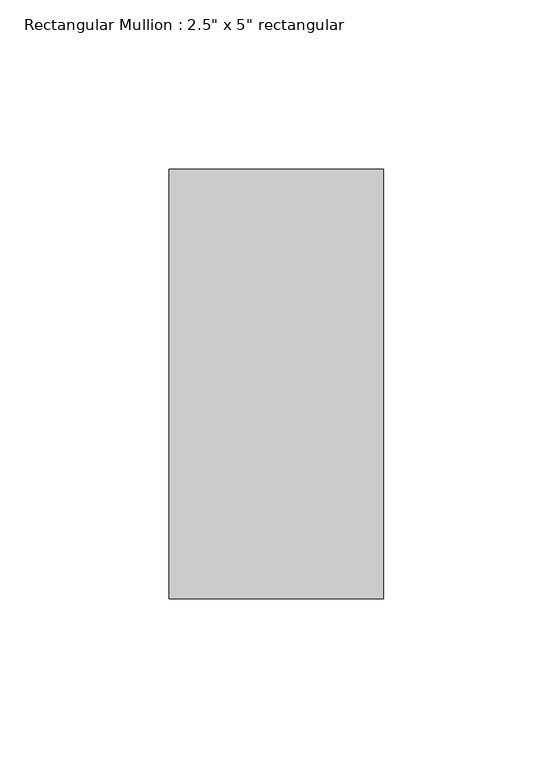
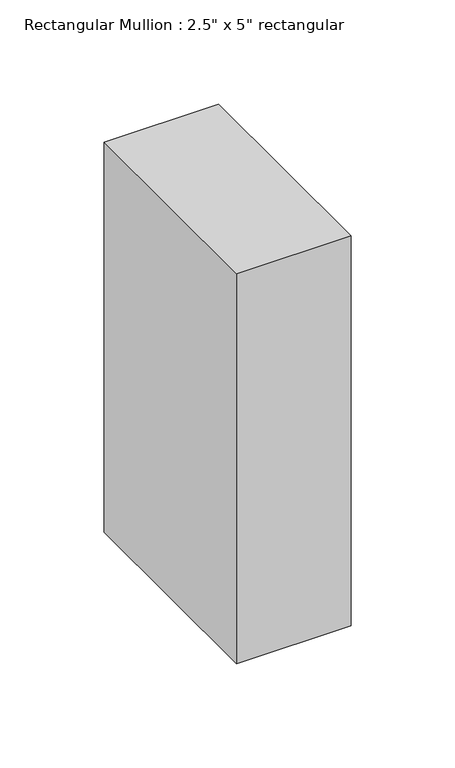
"""IFC4 building model written with IfcOpenShell, lengths in millimetres: member geometry."""

from ifc_helpers import new_model, si_unit, frame, origin, place, context, project, spatial, polyline, outline, extrude, source, transform, mapped, element, save


def member_120d0cb6(model_context):
    return source(origin(), model_context, "Body", "SweptSolid", [
        extrude(outline(polyline([(0.0, 63.5), (0.0, -63.5), (-63.5, -63.5), (-63.5, 63.5), (0.0, 63.5)])), frame((0.0, 0.0, -228.6), z_axis=(0.0, 0.0, 1.0), x_axis=(1.0, 0.0, 0.0)), (0.0, 0.0, 1.0), 228.6),
    ])


if __name__ == "__main__":
    model = new_model("IFC4")
    model_context = context("Model", 3, world=origin())
    ifc_project = project(units=[si_unit("LENGTHUNIT", "METRE", prefix="MILLI")], contexts=[model_context])
    site = spatial("IfcSite", under=ifc_project)
    building = spatial("IfcBuilding", under=site)
    placement = place(None, origin())
    member_shape = member_120d0cb6(model_context)
    element("IfcMember", 1, ObjectType="Rectangular Mullion : 2.5\" x 5\" rectangular", at=placement, inside=building, context=model_context, shape_type="MappedRepresentation", body=[
        mapped(member_shape, transform((0.0, 0.0, 0.0), x_axis=(1.0, 0.0, 0.0), y_axis=(0.0, 1.0, 0.0), z_axis=(0.0, 0.0, 1.0))),
    ])
    save(model, "model.ifc")

# Revit data of these elements
# Type "Rectangular Mullion : 2.5\" x 5\" rectangular"
#   built-in parameter 1007304 = 0.416667 (stored number, unit not read)
#   built-in parameter 1007301 = 0.104167 (stored number, unit not read)
#   built-in parameter 1007300 = 0.104167 (stored number, unit not read)
# Element 1 (IfcMember, "Rectangular Mullion : 2.5\" x 5\" rectangular")
#   Materials on its faces: "Aluminum"
# Materials
#   "Aluminum": class "Metal", colour RGB 247 247 247, transparency 0, Description = "Aluminum 6061", Cost = 0
